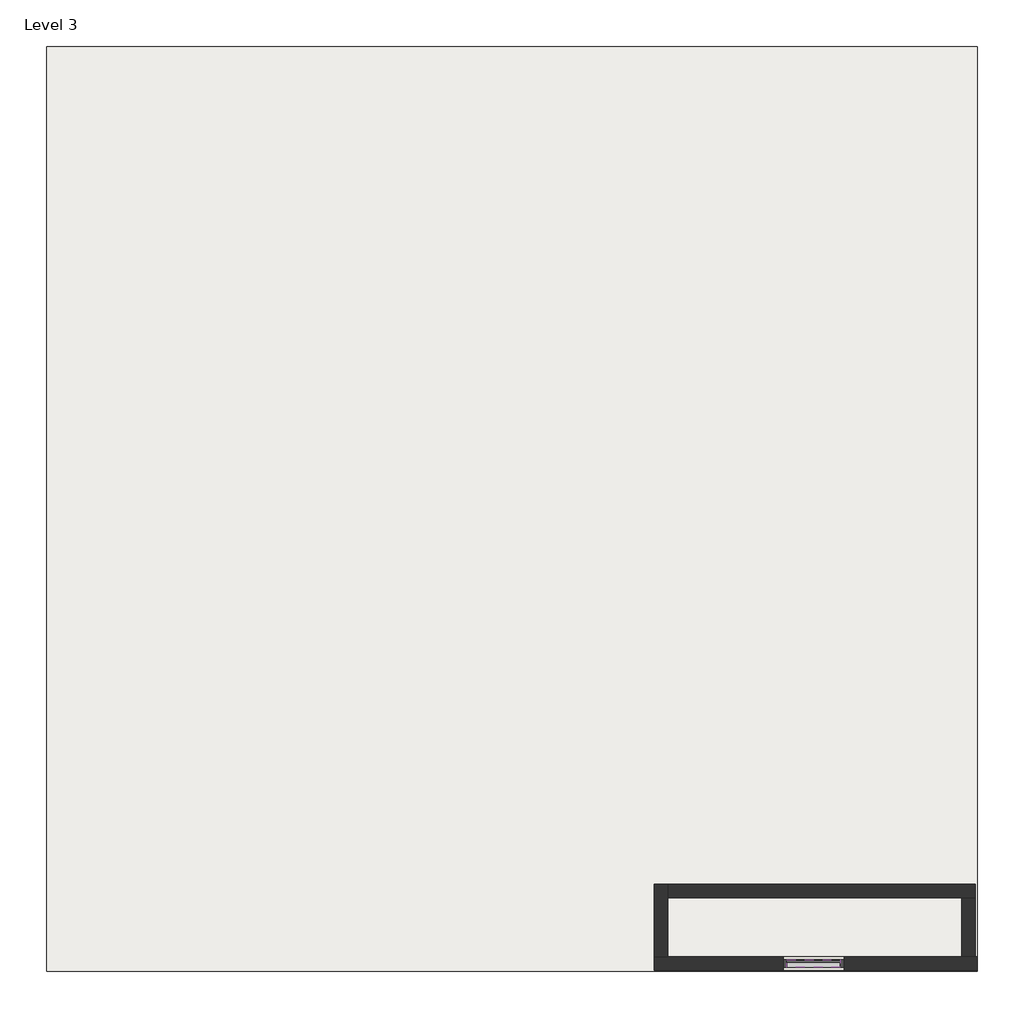
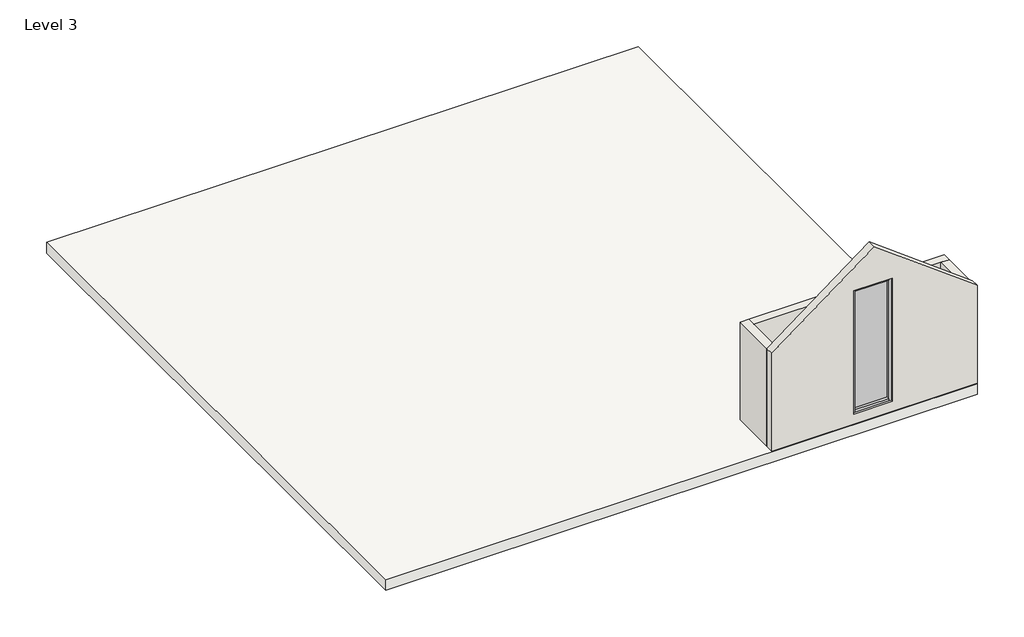
# One storey: 4 members, 4 walls, 1 plate, 1 roof.
"""IFC4 building model written with IfcOpenShell, lengths in millimetres."""

from ifc_helpers import new_model, si_unit, frame, origin, place, context, project, spatial, polyline, outline, extrude, faceted_brep, transform, mapped, element, save
from components import member_b7368e82, member_9c8919e3, system_panel_glazed_51964df0

model = new_model("IFC4")

# Units and contexts
model_context = context("Model", 3, world=origin())
ifc_project = project(units=[si_unit("LENGTHUNIT", "METRE", prefix="MILLI")], contexts=[model_context])

# Site, building, storey
site = spatial("IfcSite", under=ifc_project)
building = spatial("IfcBuilding", under=site)
storey = spatial("IfcBuildingStorey", under=building, Name="Level 3", Elevation=6096.0)

# Members
placement = place(None, origin())
member_shape = member_b7368e82(model_context)
element("IfcMember", 1, ObjectType="Rectangular Mullion : 2.5\" x 5\" rectangular", at=placement, inside=storey, context=model_context, shape_type="MappedRepresentation", body=[
    mapped(member_shape, transform((-5936.514323, -13733.5515716, 10137.3622598), x_axis=(0.0, 0.0, 1.0), y_axis=(0.0, -1.0, 0.0), z_axis=(1.0, 0.0, 0.0))),
])
element("IfcMember", 2, ObjectType="Rectangular Mullion : 2.5\" x 5\" rectangular", at=placement, inside=storey, context=model_context, shape_type="MappedRepresentation", body=[
    mapped(member_shape, transform((-6838.214323, -13733.5515716, 6682.7521998), x_axis=(0.0, 0.0, -1.0), y_axis=(0.0, -1.0, 0.0), z_axis=(-1.0, 0.0, 0.0))),
])
member_2_shape = member_9c8919e3(model_context)
element("IfcMember", 3, ObjectType="Rectangular Mullion : 2.5\" x 5\" rectangular", at=placement, inside=storey, context=model_context, shape_type="MappedRepresentation", body=[
    mapped(member_2_shape, transform((-6901.714323, -13733.5515716, 10137.3622598), x_axis=(-1.0, 0.0, 0.0), y_axis=(0.0, -1.0, 0.0), z_axis=(0.0, 0.0, 1.0))),
])
element("IfcMember", 4, ObjectType="Rectangular Mullion : 2.5\" x 5\" rectangular", at=placement, inside=storey, context=model_context, shape_type="MappedRepresentation", body=[
    mapped(member_2_shape, transform((-5873.014323, -13733.5515716, 6682.7521998), x_axis=(1.0, 0.0, 0.0), y_axis=(0.0, -1.0, 0.0), z_axis=(0.0, 0.0, -1.0))),
])

# Plate
system_panel_glazed_shape = system_panel_glazed_51964df0(model_context)
element("IfcPlate", 5, ObjectType="System Panel : Glazed", at=placement, inside=storey, context=model_context, shape_type="MappedRepresentation", body=[
    mapped(system_panel_glazed_shape, transform((-6387.364323, -13733.5515716, 6746.2521998), x_axis=(1.0, 0.0, 0.0), y_axis=(0.0, 1.0, 0.0), z_axis=(0.0, 0.0, 1.0))),
])

# Roof
element("IfcRoof", 6, ObjectType="Generic - 12\"", at=placement, inside=storey, context=model_context, shape_type="SweptSolid", body=[
    extrude(outline(polyline([(-19322.314323, 1728.7461837), (-3625.114323, 1728.7461837), (-3625.114323, -13864.3466243), (-19322.314323, -13864.3466243), (-19322.314323, 1728.7461837)])), frame((0.0, 0.0, 6096.0), z_axis=(0.0, 0.0, 1.0), x_axis=(1.0, 0.0, 0.0)), (0.0, 0.0, 1.0), 304.8),
])

# Walls
element("IfcWall", 7, ObjectType="9\"", at=placement, inside=storey, context=model_context, shape_type="Brep", body=[
    faceted_brep([(-3625.114323, -13619.2515716, 6096.0), (-3663.214323, -13619.2515716, 6096.0), (-3891.814323, -13619.2515716, 6096.0), (-8844.814323, -13619.2515716, 6096.0), (-9073.414323, -13619.2515716, 6096.0), (-9073.414323, -13619.2515716, 9144.0), (-6349.264323, -13619.2515716, 11187.1125), (-3625.114323, -13619.2515716, 9144.0), (-6901.714323, -13619.2515716, 10137.3622598), (-6901.714323, -13619.2515716, 6682.7521998), (-5873.014323, -13619.2515716, 6682.7521998), (-5873.014323, -13619.2515716, 10137.3622598), (-9073.414323, -13847.8515716, 6096.0), (-3625.114323, -13847.8515716, 6096.0), (-3625.114323, -13847.8515716, 9144.0), (-6349.264323, -13847.8515716, 11187.1125), (-9073.414323, -13847.8515716, 9144.0), (-6901.714323, -13847.8515716, 6682.7521998), (-6901.714323, -13847.8515716, 10137.3622598), (-5873.014323, -13847.8515716, 10137.3622598), (-5873.014323, -13847.8515716, 6682.7521998)], [[[0, 1, 2, 3, 4, 5, 6, 7], [8, 9, 10, 11]], [[12, 13, 14, 15, 16], [17, 18, 19, 20]], [[4, 3, 2, 1, 0, 13, 12]], [[0, 7, 14, 13]], [[5, 4, 12, 16]], [[14, 7, 6, 15]], [[5, 16, 15, 6]], [[17, 9, 8, 18]], [[18, 8, 11, 19]], [[19, 11, 10, 20]], [[9, 17, 20, 10]]]),
])
element("IfcWall", 8, ObjectType="9\"", at=placement, inside=storey, context=model_context, shape_type="Brep", body=[
    faceted_brep([(-8844.814323, -13619.2515716, 6096.0), (-8844.814323, -12628.6515716, 6096.0), (-8844.814323, -12400.0515716, 6096.0), (-8844.814323, -12400.0515716, 9144.0), (-8844.814323, -12628.6515716, 9144.0), (-8844.814323, -13619.2515716, 9144.0), (-9073.414323, -13619.2515716, 6096.0), (-9073.414323, -13619.2515716, 9144.0), (-9073.414323, -12400.0515716, 9144.0), (-9073.414323, -12400.0515716, 6096.0)], [[[0, 1, 2, 3, 4, 5]], [[6, 7, 8, 9]], [[2, 1, 0, 6, 9]], [[5, 4, 3, 8, 7]], [[0, 5, 7, 6]], [[3, 2, 9, 8]]]),
])
element("IfcWall", 9, ObjectType="9\"", at=placement, inside=storey, context=model_context, shape_type="Brep", body=[
    faceted_brep([(-8844.814323, -12628.6515716, 6096.0), (-3891.814323, -12628.6515716, 6096.0), (-3663.214323, -12628.6515716, 6096.0), (-3663.214323, -12628.6515716, 9144.0), (-3891.814323, -12628.6515716, 9144.0), (-8844.814323, -12628.6515716, 9144.0), (-8844.814323, -12400.0515716, 6096.0), (-8844.814323, -12400.0515716, 9144.0), (-3663.214323, -12400.0515716, 9144.0), (-3663.214323, -12400.0515716, 6096.0)], [[[0, 1, 2, 3, 4, 5]], [[6, 7, 8, 9]], [[2, 1, 0, 6, 9]], [[5, 4, 3, 8, 7]], [[0, 5, 7, 6]], [[3, 2, 9, 8]]]),
])
element("IfcWall", 10, ObjectType="9\"", at=placement, inside=storey, context=model_context, shape_type="SweptSolid", body=[
    extrude(outline(polyline([(-3891.814323, -13619.2515716), (-3891.814323, -12628.6515716), (-3663.214323, -12628.6515716), (-3663.214323, -13619.2515716), (-3891.814323, -13619.2515716)])), frame((0.0, 0.0, 6096.0), z_axis=(0.0, 0.0, 1.0), x_axis=(1.0, 0.0, 0.0)), (0.0, 0.0, 1.0), 3048.0),
])

save(model, "model.ifc")

# Revit data of these elements
# Type "Rectangular Mullion : 2.5\" x 5\" rectangular"
#   built-in parameter 1007304 = 0.416667 (stored number, unit not read)
#   built-in parameter 1007301 = 0.104167 (stored number, unit not read)
#   built-in parameter 1007300 = 0.104167 (stored number, unit not read)
# Type "System Panel : Glazed"
#   Construction Type Id = "GSP4R"
#   Analytic Construction = "1/8 in Pilkington single glazing"
#   Visual Light Transmittance = 0.9
#   Solar Heat Gain Coefficient = 0.86
#   Heat Transfer Coefficient (U) = 1.18115 BTU/(h·ft²·°F)
#   Define Thermal Properties by = 1
# Type "Generic - 12\""
#   Assembly Code = "B1020"
#   Layers, outside or top first: 1' - 0" no material (function 1)
# Type "9\""
#   Assembly Code = "B2010"
#   Layers, outside or top first: 0' - 9" no material (function 1)
# Elements 1, 2, 3, 4 (IfcMember, "Rectangular Mullion : 2.5\" x 5\" rectangular")
#   Phase Created = New Construction
#   Materials on its faces: "Aluminum"
# Element 5 (IfcPlate, "System Panel : Glazed")
#   Phase Created = New Construction
#   Materials on its faces: "Glass"
# Element 6 (IfcRoof, "Generic - 12\"")
#   built-in parameter 1001705 = 21 (stored number, unit not read)
#   built-in parameter 1001710 = 33615
#   Phase Created = New Construction
#   Materials on its faces: "Default Roof"
# Elements 7, 8, 9, 10 (IfcWall, "9\"")
#   Top Offset = 0' - 0"
#   Base Offset = 0' - 0"
#   Unconnected Height = 10' - 0"
#   wall height = 10' - 0"
#   Phase Created = New Construction
#   Base Constraint = Level 3
#   Materials on its faces: "Default Wall"
# Materials
#   "Aluminum": class "Metal", colour RGB 247 247 247, transparency 0, Description = "Aluminum 6061", Cost = 0
#   "Glass": class "Glass", colour RGB 0 128 192, transparency 0.75, Description = "Soda Lime Glass", Cost = 0
#   "Default Roof": colour RGB 88 101 114, transparency 0, Cost = 0
#   "Default Wall": colour RGB 128 128 128, transparency 0, Cost = 0
